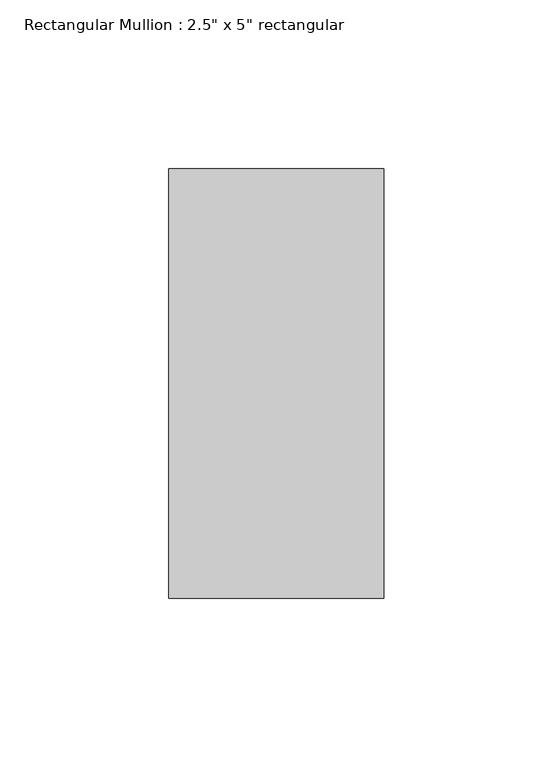
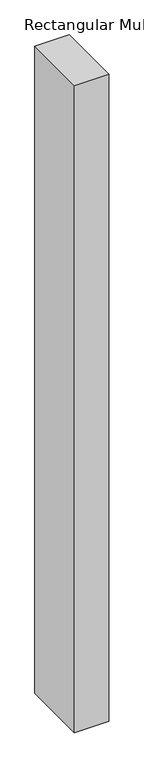
"""IFC4 building model written with IfcOpenShell, lengths in millimetres: member geometry."""

from ifc_helpers import new_model, si_unit, frame, origin, place, context, project, spatial, polyline, outline, extrude, source, transform, mapped, element, save


def member_eb359e9e(model_context):
    return source(origin(), model_context, "Body", "SweptSolid", [
        extrude(outline(polyline([(0.0, 63.5), (0.0, -63.5), (-63.5, -63.5), (-63.5, 63.5), (0.0, 63.5)])), frame((0.0, 0.0, -1267.8833333), z_axis=(0.0, 0.0, 1.0), x_axis=(1.0, 0.0, 0.0)), (0.0, 0.0, 1.0), 1267.8833333),
    ])


if __name__ == "__main__":
    model = new_model("IFC4")
    model_context = context("Model", 3, world=origin())
    ifc_project = project(units=[si_unit("LENGTHUNIT", "METRE", prefix="MILLI")], contexts=[model_context])
    site = spatial("IfcSite", under=ifc_project)
    building = spatial("IfcBuilding", under=site)
    placement = place(None, origin())
    member_shape = member_eb359e9e(model_context)
    element("IfcMember", 1, ObjectType="Rectangular Mullion : 2.5\" x 5\" rectangular", at=placement, inside=building, context=model_context, shape_type="MappedRepresentation", body=[
        mapped(member_shape, transform((0.0, 0.0, 0.0), x_axis=(1.0, 0.0, 0.0), y_axis=(0.0, 1.0, 0.0), z_axis=(0.0, 0.0, 1.0))),
    ])
    save(model, "model.ifc")

# Revit data of these elements
# Type "Rectangular Mullion : 2.5\" x 5\" rectangular"
#   built-in parameter 1007304 = 0.416667 (stored number, unit not read)
#   built-in parameter 1007301 = 0.104167 (stored number, unit not read)
#   built-in parameter 1007300 = 0.104167 (stored number, unit not read)
# Element 1 (IfcMember, "Rectangular Mullion : 2.5\" x 5\" rectangular")
#   Materials on its faces: "Aluminum"
# Materials
#   "Aluminum": class "Metal", colour RGB 247 247 247, transparency 0, Description = "Aluminum 6061", Cost = 0
